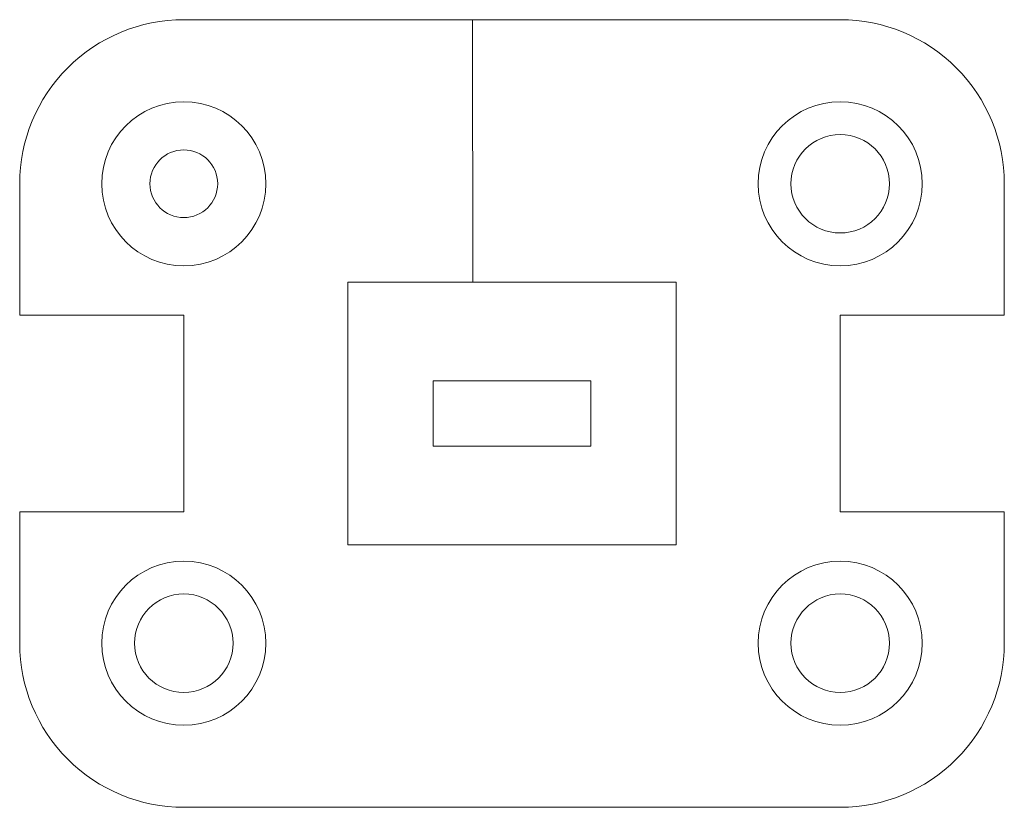
# Model space of a CAD drawing. Units: millimetres. Extents: x 0 to 2069, y 995 to 1695.
# Tile 2 of 2: x 1919 to 2069, y 995 to 1115. Entities that reach past the tile are written whole.
import ezdxf

# ---------------------------------------------------------------- set-up
doc = ezdxf.new("R2010")
doc.units = ezdxf.units.MM
doc.layers.add('M-CONS', color=8, linetype='Continuous', lineweight=18)

msp = doc.modelspace()

# ---------------------------------------------------------------- linework, layer by layer
at = {"layer": 'M-CONS', "extrusion": (0, 1, 0)}
for p, q in [((1993.94, 1115.06, 15), (1987.94, 1115.06, 15)), ((1987.94, 1115.06, 15), (1987.97, 1075.06, 64.28)), ((2018.94, 1075.06, 40), (1968.94, 1075.06, 40)), ((1993.94, 1075.06, 40), (1987.94, 1075.06, 40)), ((1987.97, 1075.06, 61.62), (1987.97, 1075.06, 64.28)), ((1993.94, 1075.06, 65), (1993.94, 1075.06, 65)), ((1999.97, 1075.06, 61.61), (1999.97, 1075.06, 64.26))]:
    msp.add_line(p, q, dxfattribs=at)
at = {"layer": 'M-CONS'}
for p, q in [((2018.94, 1055.06), (2018.94, 1061.46)), ((2005.94, 1055.06), (2005.94, 1060.06)), ((1968.94, 1055.06), (1968.94, 1042.74))]:
    msp.add_line(p, q, dxfattribs=at)
for points in [[(2068.94, 1090.06), (2068.94, 1070.06), (2068.94, 1090.06, 0.414214), (2043.94, 1115.06), (1943.94, 1115.06, 0.414214), (1918.94, 1090.06), (1918.94, 1070.06), (1943.94, 1070.06), (1943.94, 1055.06)], [(2068.94, 1070.06), (2043.94, 1070.06), (2043.94, 1040.06), (2068.94, 1040.06), (2068.94, 1020.06, -0.414214), (2043.94, 995.06), (1943.94, 995.06, -0.414214), (1918.94, 1020.06), (1918.94, 1040.06), (1943.94, 1040.06), (1943.94, 1070.06)]]:
    msp.add_lwpolyline(points, format="xyb", dxfattribs=at)
for points in [[(1968.94, 1035.06), (1968.94, 1075.06), (2018.94, 1075.06), (2018.94, 1035.06)], [(1981.94, 1060.06), (1981.94, 1050.06), (2005.94, 1050.06), (2005.94, 1060.06)]]:
    msp.add_lwpolyline(points, close=True, dxfattribs=at)
at = {"layer": 'M-CONS', "extrusion": (0, -1, 0), "elevation": -1035.06}
msp.add_lwpolyline([(1981.44, 40), (1968.94, 40, -1), (2018.94, 40), (2006.44, 40)], format="xyb", dxfattribs=at)
at = {"layer": 'M-CONS'}
for centre, radius in [((1943.94, 1090.06), 12.5), ((2043.94, 1090.06), 12.5), ((2043.94, 1090.06), 7.5), ((1943.94, 1090.06), 5.16), ((1943.94, 1020.06), 12.5), ((2043.94, 1020.06), 12.5), ((1943.94, 1020.06), 7.5), ((2043.94, 1020.06), 7.5)]:
    msp.add_circle(centre, radius, dxfattribs=at)
at = {"layer": 'M-CONS', "extrusion": (0, -1, 0)}
msp.add_circle((1993.94, 40, -1035.06), 12.5, dxfattribs=at)
msp.add_circle((1993.94, 40, -1035.06), 12.5, dxfattribs=at)

doc.saveas('drawing.dxf')
